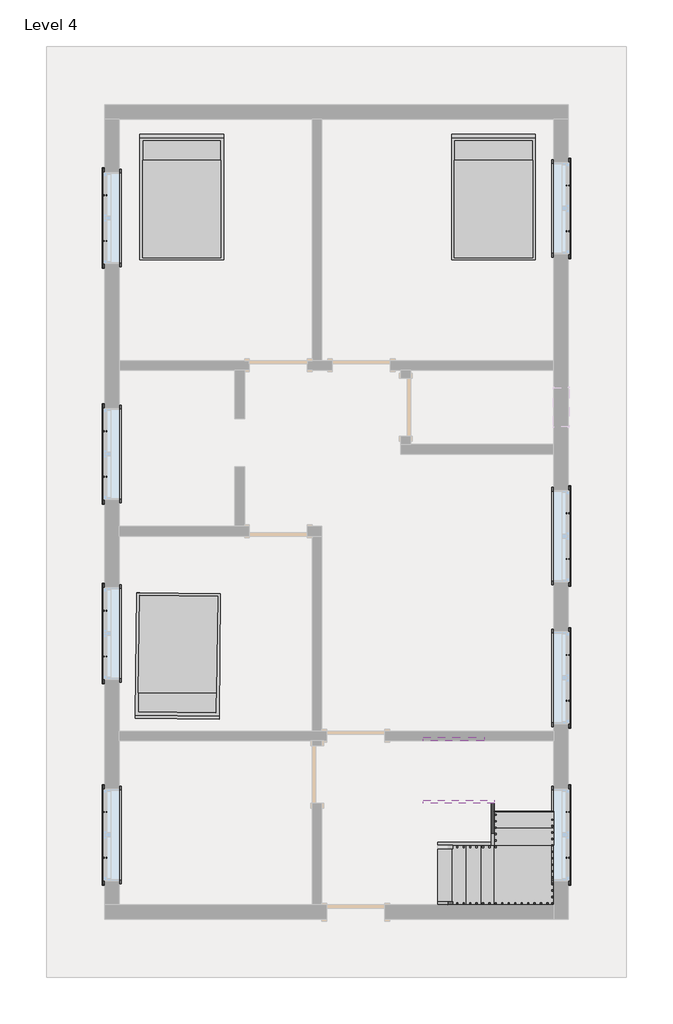
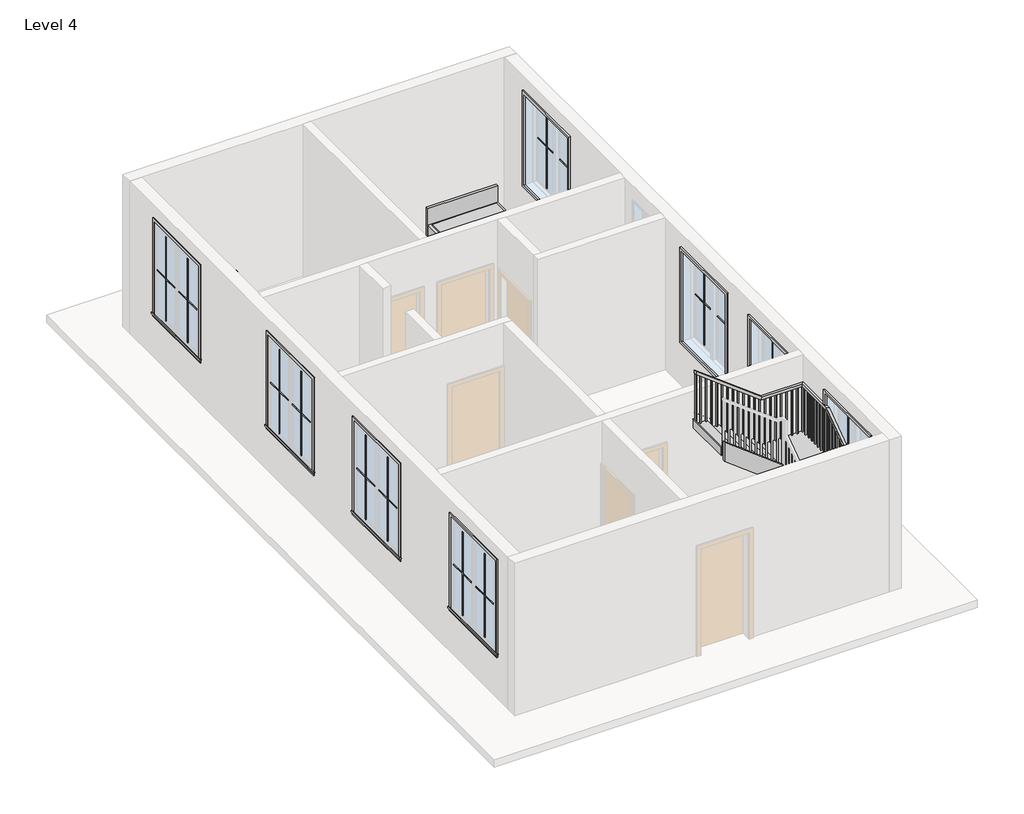
# One storey, part 2 of 2: 32 proxies, 5 members, 3 furniture elements, 1 railing, 1 stair flight.
"""IFC4 building model written with IfcOpenShell, lengths in millimetres."""

from ifc_helpers import new_model, si_unit, frame, origin, place, context, project, spatial, polyline, outline, extrude, faceted_brep, transform, mapped, element, save
from components import muntin_pattern_2x2_muntin_pattern_2x2_bff912c5, muntin_pattern_2x2_muntin_pattern_2x2_c2194282, trim_window_exterior_flat_with_sill_e04b3088, trim_window_interior_flat_picture_frame_2a7685fe, bed_17739_bed_17739_15c61121, stair_flight_c7955c98

model = new_model("IFC4")

# Units and contexts
model_context = context("Model", 3, world=origin())
ifc_project = project(units=[si_unit("LENGTHUNIT", "METRE", prefix="MILLI")], contexts=[model_context])

# Site, building, storey
site = spatial("IfcSite", under=ifc_project)
building = spatial("IfcBuilding", under=site)
storey = spatial("IfcBuildingStorey", under=building, Name="Level 4", Elevation=6400.8)

# Proxies
placement = place(None, origin())
muntin_pattern_2x2_muntin_pattern_2x2_shape = muntin_pattern_2x2_muntin_pattern_2x2_bff912c5(model_context)
element("IfcBuildingElementProxy", 1, Name="Muntin Pattern_2x2 : Muntin Pattern_2x2", ObjectType="Muntin Pattern_2x2 : Muntin Pattern_2x2", at=placement, inside=storey, context=model_context, shape_type="MappedRepresentation", body=[
    mapped(muntin_pattern_2x2_muntin_pattern_2x2_shape, transform((-4903.510885, -5396.5975571, 7385.05), x_axis=(0.0, 1.0, 0.0), y_axis=(-1.0, 0.0, 0.0), z_axis=(0.0, 0.0, 1.0))),
])
element("IfcBuildingElementProxy", 2, Name="Muntin Pattern_2x2 : Muntin Pattern_2x2", ObjectType="Muntin Pattern_2x2 : Muntin Pattern_2x2", at=placement, inside=storey, context=model_context, shape_type="MappedRepresentation", body=[
    mapped(muntin_pattern_2x2_muntin_pattern_2x2_shape, transform((2392.639115, -4675.8725571, 7385.05), x_axis=(0.0, -1.0, 0.0), y_axis=(1.0, 0.0, 0.0), z_axis=(0.0, 0.0, 1.0))),
])
element("IfcBuildingElementProxy", 3, Name="Muntin Pattern_2x2 : Muntin Pattern_2x2", ObjectType="Muntin Pattern_2x2 : Muntin Pattern_2x2", at=placement, inside=storey, context=model_context, shape_type="MappedRepresentation", body=[
    mapped(muntin_pattern_2x2_muntin_pattern_2x2_shape, transform((2392.639115, -2199.3725571, 7385.05), x_axis=(0.0, -1.0, 0.0), y_axis=(1.0, 0.0, 0.0), z_axis=(0.0, 0.0, 1.0))),
])
element("IfcBuildingElementProxy", 4, Name="Muntin Pattern_2x2 : Muntin Pattern_2x2", ObjectType="Muntin Pattern_2x2 : Muntin Pattern_2x2", at=placement, inside=storey, context=model_context, shape_type="MappedRepresentation", body=[
    mapped(muntin_pattern_2x2_muntin_pattern_2x2_shape, transform((2392.639115, 35.8274429, 7385.05), x_axis=(0.0, -1.0, 0.0), y_axis=(1.0, 0.0, 0.0), z_axis=(0.0, 0.0, 1.0))),
])
element("IfcBuildingElementProxy", 5, Name="Muntin Pattern_2x2 : Muntin Pattern_2x2", ObjectType="Muntin Pattern_2x2 : Muntin Pattern_2x2", at=placement, inside=storey, context=model_context, shape_type="MappedRepresentation", body=[
    mapped(muntin_pattern_2x2_muntin_pattern_2x2_shape, transform((-4903.510885, -2221.5975571, 7385.05), x_axis=(0.0, 1.0, 0.0), y_axis=(-1.0, 0.0, 0.0), z_axis=(0.0, 0.0, 1.0))),
])
element("IfcBuildingElementProxy", 6, Name="Muntin Pattern_2x2 : Muntin Pattern_2x2", ObjectType="Muntin Pattern_2x2 : Muntin Pattern_2x2", at=placement, inside=storey, context=model_context, shape_type="MappedRepresentation", body=[
    mapped(muntin_pattern_2x2_muntin_pattern_2x2_shape, transform((-4903.510885, 610.5024429, 7385.05), x_axis=(0.0, 1.0, 0.0), y_axis=(-1.0, 0.0, 0.0), z_axis=(0.0, 0.0, 1.0))),
])
element("IfcBuildingElementProxy", 7, Name="Muntin Pattern_2x2 : Muntin Pattern_2x2", ObjectType="Muntin Pattern_2x2 : Muntin Pattern_2x2", at=placement, inside=storey, context=model_context, shape_type="MappedRepresentation", body=[
    mapped(muntin_pattern_2x2_muntin_pattern_2x2_shape, transform((-4903.510885, 4331.6024429, 7385.05), x_axis=(0.0, 1.0, 0.0), y_axis=(-1.0, 0.0, 0.0), z_axis=(0.0, 0.0, 1.0))),
])
element("IfcBuildingElementProxy", 8, Name="Muntin Pattern_2x2 : Muntin Pattern_2x2", ObjectType="Muntin Pattern_2x2 : Muntin Pattern_2x2", at=placement, inside=storey, context=model_context, shape_type="MappedRepresentation", body=[
    mapped(muntin_pattern_2x2_muntin_pattern_2x2_shape, transform((2392.639115, 5204.7274429, 7385.05), x_axis=(0.0, -1.0, 0.0), y_axis=(1.0, 0.0, 0.0), z_axis=(0.0, 0.0, 1.0))),
])
muntin_pattern_2x2_muntin_pattern_2x2_2_shape = muntin_pattern_2x2_muntin_pattern_2x2_c2194282(model_context)
element("IfcBuildingElementProxy", 9, Name="Muntin Pattern_2x2 : Muntin Pattern_2x2", ObjectType="Muntin Pattern_2x2 : Muntin Pattern_2x2", at=placement, inside=storey, context=model_context, shape_type="MappedRepresentation", body=[
    mapped(muntin_pattern_2x2_muntin_pattern_2x2_2_shape, transform((-4903.510885, -4675.8725571, 7385.05), x_axis=(0.0, -1.0, 0.0), y_axis=(1.0, 0.0, 0.0), z_axis=(0.0, 0.0, 1.0))),
])
element("IfcBuildingElementProxy", 10, Name="Muntin Pattern_2x2 : Muntin Pattern_2x2", ObjectType="Muntin Pattern_2x2 : Muntin Pattern_2x2", at=placement, inside=storey, context=model_context, shape_type="MappedRepresentation", body=[
    mapped(muntin_pattern_2x2_muntin_pattern_2x2_2_shape, transform((2392.639115, -5396.5975571, 7385.05), x_axis=(0.0, 1.0, 0.0), y_axis=(-1.0, 0.0, 0.0), z_axis=(0.0, 0.0, 1.0))),
])
element("IfcBuildingElementProxy", 11, Name="Muntin Pattern_2x2 : Muntin Pattern_2x2", ObjectType="Muntin Pattern_2x2 : Muntin Pattern_2x2", at=placement, inside=storey, context=model_context, shape_type="MappedRepresentation", body=[
    mapped(muntin_pattern_2x2_muntin_pattern_2x2_2_shape, transform((2392.639115, -2920.0975571, 7385.05), x_axis=(0.0, 1.0, 0.0), y_axis=(-1.0, 0.0, 0.0), z_axis=(0.0, 0.0, 1.0))),
])
element("IfcBuildingElementProxy", 12, Name="Muntin Pattern_2x2 : Muntin Pattern_2x2", ObjectType="Muntin Pattern_2x2 : Muntin Pattern_2x2", at=placement, inside=storey, context=model_context, shape_type="MappedRepresentation", body=[
    mapped(muntin_pattern_2x2_muntin_pattern_2x2_2_shape, transform((2392.639115, -684.8975571, 7385.05), x_axis=(0.0, 1.0, 0.0), y_axis=(-1.0, 0.0, 0.0), z_axis=(0.0, 0.0, 1.0))),
])
element("IfcBuildingElementProxy", 13, Name="Muntin Pattern_2x2 : Muntin Pattern_2x2", ObjectType="Muntin Pattern_2x2 : Muntin Pattern_2x2", at=placement, inside=storey, context=model_context, shape_type="MappedRepresentation", body=[
    mapped(muntin_pattern_2x2_muntin_pattern_2x2_2_shape, transform((-4903.510885, -1500.8725571, 7385.05), x_axis=(0.0, -1.0, 0.0), y_axis=(1.0, 0.0, 0.0), z_axis=(0.0, 0.0, 1.0))),
])
element("IfcBuildingElementProxy", 14, Name="Muntin Pattern_2x2 : Muntin Pattern_2x2", ObjectType="Muntin Pattern_2x2 : Muntin Pattern_2x2", at=placement, inside=storey, context=model_context, shape_type="MappedRepresentation", body=[
    mapped(muntin_pattern_2x2_muntin_pattern_2x2_2_shape, transform((-4903.510885, 1331.2274429, 7385.05), x_axis=(0.0, -1.0, 0.0), y_axis=(1.0, 0.0, 0.0), z_axis=(0.0, 0.0, 1.0))),
])
element("IfcBuildingElementProxy", 15, Name="Muntin Pattern_2x2 : Muntin Pattern_2x2", ObjectType="Muntin Pattern_2x2 : Muntin Pattern_2x2", at=placement, inside=storey, context=model_context, shape_type="MappedRepresentation", body=[
    mapped(muntin_pattern_2x2_muntin_pattern_2x2_2_shape, transform((-4903.510885, 5052.3274429, 7385.05), x_axis=(0.0, -1.0, 0.0), y_axis=(1.0, 0.0, 0.0), z_axis=(0.0, 0.0, 1.0))),
])
element("IfcBuildingElementProxy", 16, Name="Muntin Pattern_2x2 : Muntin Pattern_2x2", ObjectType="Muntin Pattern_2x2 : Muntin Pattern_2x2", at=placement, inside=storey, context=model_context, shape_type="MappedRepresentation", body=[
    mapped(muntin_pattern_2x2_muntin_pattern_2x2_2_shape, transform((2392.639115, 4484.0024429, 7385.05), x_axis=(0.0, 1.0, 0.0), y_axis=(-1.0, 0.0, 0.0), z_axis=(0.0, 0.0, 1.0))),
])
trim_window_exterior_flat_with_sill_shape = trim_window_exterior_flat_with_sill_e04b3088(model_context)
element("IfcBuildingElementProxy", 17, Name="Trim-Window-Exterior-Flat : with Sill", ObjectType="Trim-Window-Exterior-Flat : with Sill", at=placement, inside=storey, context=model_context, shape_type="MappedRepresentation", body=[
    mapped(trim_window_exterior_flat_with_sill_shape, transform((-4913.035885, -5036.2350571, 9144.0), x_axis=(0.0, -1.0, 0.0), y_axis=(0.0, 0.0, 1.0), z_axis=(-1.0, 0.0, 0.0))),
])
element("IfcBuildingElementProxy", 18, Name="Trim-Window-Exterior-Flat : with Sill", ObjectType="Trim-Window-Exterior-Flat : with Sill", at=placement, inside=storey, context=model_context, shape_type="MappedRepresentation", body=[
    mapped(trim_window_exterior_flat_with_sill_shape, transform((2402.164115, -5036.2350571, 9144.0), x_axis=(0.0, 1.0, 0.0), y_axis=(0.0, 0.0, 1.0), z_axis=(1.0, 0.0, 0.0))),
])
element("IfcBuildingElementProxy", 19, Name="Trim-Window-Exterior-Flat : with Sill", ObjectType="Trim-Window-Exterior-Flat : with Sill", at=placement, inside=storey, context=model_context, shape_type="MappedRepresentation", body=[
    mapped(trim_window_exterior_flat_with_sill_shape, transform((2402.164115, -2559.7350571, 9144.0), x_axis=(0.0, 1.0, 0.0), y_axis=(0.0, 0.0, 1.0), z_axis=(1.0, 0.0, 0.0))),
])
element("IfcBuildingElementProxy", 20, Name="Trim-Window-Exterior-Flat : with Sill", ObjectType="Trim-Window-Exterior-Flat : with Sill", at=placement, inside=storey, context=model_context, shape_type="MappedRepresentation", body=[
    mapped(trim_window_exterior_flat_with_sill_shape, transform((2402.164115, -324.5350571, 9144.0), x_axis=(0.0, 1.0, 0.0), y_axis=(0.0, 0.0, 1.0), z_axis=(1.0, 0.0, 0.0))),
])
element("IfcBuildingElementProxy", 21, Name="Trim-Window-Exterior-Flat : with Sill", ObjectType="Trim-Window-Exterior-Flat : with Sill", at=placement, inside=storey, context=model_context, shape_type="MappedRepresentation", body=[
    mapped(trim_window_exterior_flat_with_sill_shape, transform((-4913.035885, -1861.2350571, 9144.0), x_axis=(0.0, -1.0, 0.0), y_axis=(0.0, 0.0, 1.0), z_axis=(-1.0, 0.0, 0.0))),
])
element("IfcBuildingElementProxy", 22, Name="Trim-Window-Exterior-Flat : with Sill", ObjectType="Trim-Window-Exterior-Flat : with Sill", at=placement, inside=storey, context=model_context, shape_type="MappedRepresentation", body=[
    mapped(trim_window_exterior_flat_with_sill_shape, transform((-4913.035885, 970.8649429, 9144.0), x_axis=(0.0, -1.0, 0.0), y_axis=(0.0, 0.0, 1.0), z_axis=(-1.0, 0.0, 0.0))),
])
element("IfcBuildingElementProxy", 23, Name="Trim-Window-Exterior-Flat : with Sill", ObjectType="Trim-Window-Exterior-Flat : with Sill", at=placement, inside=storey, context=model_context, shape_type="MappedRepresentation", body=[
    mapped(trim_window_exterior_flat_with_sill_shape, transform((-4913.035885, 4691.9649429, 9144.0), x_axis=(0.0, -1.0, 0.0), y_axis=(0.0, 0.0, 1.0), z_axis=(-1.0, 0.0, 0.0))),
])
element("IfcBuildingElementProxy", 24, Name="Trim-Window-Exterior-Flat : with Sill", ObjectType="Trim-Window-Exterior-Flat : with Sill", at=placement, inside=storey, context=model_context, shape_type="MappedRepresentation", body=[
    mapped(trim_window_exterior_flat_with_sill_shape, transform((2402.164115, 4844.3649429, 9144.0), x_axis=(0.0, 1.0, 0.0), y_axis=(0.0, 0.0, 1.0), z_axis=(1.0, 0.0, 0.0))),
])
trim_window_interior_flat_picture_frame_shape = trim_window_interior_flat_picture_frame_2a7685fe(model_context)
element("IfcBuildingElementProxy", 25, Name="Trim-Window-Interior-Flat : Picture Frame", ObjectType="Trim-Window-Interior-Flat : Picture Frame", at=placement, inside=storey, context=model_context, shape_type="MappedRepresentation", body=[
    mapped(trim_window_interior_flat_picture_frame_shape, transform((-4684.435885, -5036.2350571, 9144.0), x_axis=(0.0, 1.0, 0.0), y_axis=(0.0, 0.0, 1.0), z_axis=(1.0, 0.0, 0.0))),
])
element("IfcBuildingElementProxy", 26, Name="Trim-Window-Interior-Flat : Picture Frame", ObjectType="Trim-Window-Interior-Flat : Picture Frame", at=placement, inside=storey, context=model_context, shape_type="MappedRepresentation", body=[
    mapped(trim_window_interior_flat_picture_frame_shape, transform((2173.564115, -5036.2350571, 9144.0), x_axis=(0.0, -1.0, 0.0), y_axis=(0.0, 0.0, 1.0), z_axis=(-1.0, 0.0, 0.0))),
])
element("IfcBuildingElementProxy", 27, Name="Trim-Window-Interior-Flat : Picture Frame", ObjectType="Trim-Window-Interior-Flat : Picture Frame", at=placement, inside=storey, context=model_context, shape_type="MappedRepresentation", body=[
    mapped(trim_window_interior_flat_picture_frame_shape, transform((2173.564115, -2559.7350571, 9144.0), x_axis=(0.0, -1.0, 0.0), y_axis=(0.0, 0.0, 1.0), z_axis=(-1.0, 0.0, 0.0))),
])
element("IfcBuildingElementProxy", 28, Name="Trim-Window-Interior-Flat : Picture Frame", ObjectType="Trim-Window-Interior-Flat : Picture Frame", at=placement, inside=storey, context=model_context, shape_type="MappedRepresentation", body=[
    mapped(trim_window_interior_flat_picture_frame_shape, transform((2173.564115, -324.5350571, 9144.0), x_axis=(0.0, -1.0, 0.0), y_axis=(0.0, 0.0, 1.0), z_axis=(-1.0, 0.0, 0.0))),
])
element("IfcBuildingElementProxy", 29, Name="Trim-Window-Interior-Flat : Picture Frame", ObjectType="Trim-Window-Interior-Flat : Picture Frame", at=placement, inside=storey, context=model_context, shape_type="MappedRepresentation", body=[
    mapped(trim_window_interior_flat_picture_frame_shape, transform((-4684.435885, -1861.2350571, 9144.0), x_axis=(0.0, 1.0, 0.0), y_axis=(0.0, 0.0, 1.0), z_axis=(1.0, 0.0, 0.0))),
])
element("IfcBuildingElementProxy", 30, Name="Trim-Window-Interior-Flat : Picture Frame", ObjectType="Trim-Window-Interior-Flat : Picture Frame", at=placement, inside=storey, context=model_context, shape_type="MappedRepresentation", body=[
    mapped(trim_window_interior_flat_picture_frame_shape, transform((-4684.435885, 970.8649429, 9144.0), x_axis=(0.0, 1.0, 0.0), y_axis=(0.0, 0.0, 1.0), z_axis=(1.0, 0.0, 0.0))),
])
element("IfcBuildingElementProxy", 31, Name="Trim-Window-Interior-Flat : Picture Frame", ObjectType="Trim-Window-Interior-Flat : Picture Frame", at=placement, inside=storey, context=model_context, shape_type="MappedRepresentation", body=[
    mapped(trim_window_interior_flat_picture_frame_shape, transform((-4684.435885, 4691.9649429, 9144.0), x_axis=(0.0, 1.0, 0.0), y_axis=(0.0, 0.0, 1.0), z_axis=(1.0, 0.0, 0.0))),
])
element("IfcBuildingElementProxy", 32, Name="Trim-Window-Interior-Flat : Picture Frame", ObjectType="Trim-Window-Interior-Flat : Picture Frame", at=placement, inside=storey, context=model_context, shape_type="MappedRepresentation", body=[
    mapped(trim_window_interior_flat_picture_frame_shape, transform((2173.564115, 4844.3649429, 9144.0), x_axis=(0.0, -1.0, 0.0), y_axis=(0.0, 0.0, 1.0), z_axis=(-1.0, 0.0, 0.0))),
])

# Furniture
bed_17739_bed_17739_shape = bed_17739_bed_17739_15c61121(model_context)
element("IfcFurniture", 33, ObjectType="Bed_17739 : Bed_17739", at=placement, inside=storey, context=model_context, shape_type="MappedRepresentation", body=[
    mapped(bed_17739_bed_17739_shape, transform((-3693.835885, 4996.7649429, 6400.8), x_axis=(1.0, 0.0, 0.0), y_axis=(0.0, 1.0, 0.0), z_axis=(0.0, 0.0, 1.0))),
])
element("IfcFurniture", 34, ObjectType="Bed_17739 : Bed_17739", at=placement, inside=storey, context=model_context, shape_type="MappedRepresentation", body=[
    mapped(bed_17739_bed_17739_shape, transform((1221.064115, 4996.7649429, 6400.8), x_axis=(1.0, 0.0, 0.0), y_axis=(0.0, 1.0, 0.0), z_axis=(0.0, 0.0, 1.0))),
])
element("IfcFurniture", 35, ObjectType="Bed_17739 : Bed_17739", at=placement, inside=storey, context=model_context, shape_type="MappedRepresentation", body=[
    mapped(bed_17739_bed_17739_shape, transform((-3756.0321663, -2189.364606, 6400.8), x_axis=(-0.9999334593473937, 0.011535895177843815, 0.0), y_axis=(-0.011535895177843815, -0.9999334593473937, 0.0), z_axis=(0.0, 0.0, 1.0))),
])

# Members
element("IfcMember", 36, ObjectType="Stringer - 2\" Width", at=placement, inside=storey, context=model_context, shape_type="SweptSolid", body=[
    extrude(outline(polyline([(6623.4959685, 344.764115), (6400.8, 344.764115), (6400.8, 555.1685253), (6883.7196844, 1182.964115), (7268.2651993, 1182.964115), (6623.4959685, 344.764115)])), frame((0.0, -5201.3350571, 0.0), z_axis=(0.0, 1.0, 0.0), x_axis=(0.0, 0.0, 1.0)), (0.0, 0.0, 1.0), 50.8),
])
element("IfcMember", 37, ObjectType="Stringer - 2\" Width", at=placement, inside=storey, context=model_context, shape_type="SweptSolid", body=[
    extrude(outline(polyline([(-5201.3350571, 7095.952716), (-5201.3350571, 7470.5225362), (-4540.9350571, 7942.2368219), (-4540.9350571, 7567.6670017), (-5201.3350571, 7095.952716)])), frame((1182.964115, 0.0, 0.0), z_axis=(1.0, 0.0, 0.0), x_axis=(0.0, 1.0, 0.0)), (0.0, 0.0, 1.0), 50.8),
])
element("IfcMember", 38, ObjectType="Stringer - 2\" Width", at=placement, inside=storey, context=model_context, shape_type="SweptSolid", body=[
    extrude(outline(polyline([(7769.9786616, 1233.764115), (8153.1668, 1233.764115), (9004.6715619, 116.164115), (8621.4834236, 116.164115), (7769.9786616, 1233.764115)])), frame((0.0, -4540.9350571, 0.0), z_axis=(0.0, 1.0, 0.0), x_axis=(0.0, 0.0, 1.0)), (0.0, 0.0, 1.0), 50.8),
])
element("IfcMember", 39, ObjectType="Stringer - 2\" Width", at=placement, inside=storey, context=model_context, shape_type="SweptSolid", body=[
    extrude(outline(polyline([(6623.4959685, 344.764115), (6400.8, 344.764115), (6400.8, 555.1685253), (6799.2368219, 1073.1363938), (6799.2368219, 573.2272245), (6623.4959685, 344.764115)])), frame((0.0, -6191.9350571, 0.0), z_axis=(0.0, 1.0, 0.0), x_axis=(0.0, 0.0, 1.0)), (0.0, 0.0, 1.0), 50.8),
])
element("IfcMember", 40, ObjectType="Stringer - 2\" Width", at=placement, inside=storey, context=model_context, shape_type="SweptSolid", body=[
    extrude(outline(polyline([(8275.2384303, 1073.5451003), (9004.6715619, 116.164115), (8621.4834236, 116.164115), (8275.2384303, 570.6106687), (8275.2384303, 1073.5451003)])), frame((0.0, -3550.3350571, 0.0), z_axis=(0.0, 1.0, 0.0), x_axis=(0.0, 0.0, 1.0)), (0.0, 0.0, 1.0), 50.8),
])

# Railing
element("IfcRailing", 41, ObjectType="Handrail - Rectangular", at=placement, inside=storey, context=model_context, shape_type="SolidModel", body=[
    faceted_brep([(344.764115, -6090.3350571, 7484.5333333), (344.764115, -6090.3350571, 7420.6686436), (344.764115, -6141.1350571, 7420.6686436), (344.764115, -6141.1350571, 7484.5333333), (1373.464115, -6090.3350571, 8268.3047619), (1390.6115203, -6090.3350571, 8217.5047619), (1390.6115203, -6141.1350571, 8217.5047619), (1373.464115, -6141.1350571, 8268.3047619), (2122.764115, -6090.3350571, 8268.3047619), (2122.764115, -6090.3350571, 8217.5047619), (2173.564115, -6141.1350571, 8217.5047619), (2173.564115, -6141.1350571, 8268.3047619), (2122.764115, -5289.3883904, 8268.3047619), (2122.764115, -5273.1087657, 8217.5047619), (2173.564115, -5273.1087657, 8217.5047619), (2173.564115, -5289.3883904, 8268.3047619), (2122.764115, -4399.3108146, 8904.0744589), (2122.764115, -4383.0311899, 8853.2744589), (2173.564115, -4383.0311899, 8853.2744589), (2173.564115, -4399.3108146, 8904.0744589), (2122.764115, -3601.1350571, 8904.0744589), (2122.764115, -3601.1350571, 8853.2744589), (2173.564115, -3550.3350571, 8853.2744589), (2173.564115, -3550.3350571, 8904.0744589), (1371.6498293, -3601.1350571, 8904.0744589), (1354.5800477, -3601.1350571, 8853.2744589), (1354.5800477, -3550.3350571, 8853.2744589), (1371.6498293, -3550.3350571, 8904.0744589), (116.164115, -3601.1350571, 9855.2), (116.164115, -3550.3350571, 9855.2), (116.164115, -3550.3350571, 9791.4683472), (116.164115, -3601.1350571, 9791.4683472)], [[[0, 1, 2, 3]], [[1, 0, 4, 5]], [[2, 1, 5, 6]], [[3, 2, 6, 7]], [[0, 3, 7, 4]], [[5, 4, 8, 9]], [[6, 5, 9, 10]], [[7, 6, 10, 11]], [[4, 7, 11, 8]], [[9, 8, 12, 13]], [[10, 9, 13, 14]], [[11, 10, 14, 15]], [[8, 11, 15, 12]], [[13, 12, 16, 17]], [[14, 13, 17, 18]], [[15, 14, 18, 19]], [[12, 15, 19, 16]], [[17, 16, 20, 21]], [[18, 17, 21, 22]], [[19, 18, 22, 23]], [[16, 19, 23, 20]], [[21, 20, 24, 25]], [[22, 21, 25, 26]], [[23, 22, 26, 27]], [[20, 23, 27, 24]], [[28, 29, 30, 31]], [[25, 24, 28, 31]], [[26, 25, 31, 30]], [[27, 26, 30, 29]], [[24, 27, 29, 28]]]),
    extrude(outline(polyline([(9707.2827412, 227.289115), (9721.7145594, 208.239115), (8771.4666667, 208.239115), (8771.4666667, 227.289115), (9707.2827412, 227.289115)])), frame((0.0, -3585.2600571, 0.0), z_axis=(0.0, 1.0, 0.0), x_axis=(0.0, 0.0, 1.0)), (0.0, 0.0, 1.0), 19.05),
    extrude(outline(polyline([(9630.3130442, 328.889115), (9644.7448624, 309.839115), (8771.4666667, 309.839115), (8771.4666667, 328.889115), (9630.3130442, 328.889115)])), frame((0.0, -3585.2600571, 0.0), z_axis=(0.0, 1.0, 0.0), x_axis=(0.0, 0.0, 1.0)), (0.0, 0.0, 1.0), 19.05),
    extrude(outline(polyline([(9553.3433472, 430.489115), (9567.7751654, 411.439115), (8602.1333333, 411.439115), (8602.1333333, 430.489115), (9553.3433472, 430.489115)])), frame((0.0, -3585.2600571, 0.0), z_axis=(0.0, 1.0, 0.0), x_axis=(0.0, 0.0, 1.0)), (0.0, 0.0, 1.0), 19.05),
    extrude(outline(polyline([(9476.3736503, 532.089115), (9490.8054685, 513.039115), (8602.1333333, 513.039115), (8602.1333333, 532.089115), (9476.3736503, 532.089115)])), frame((0.0, -3585.2600571, 0.0), z_axis=(0.0, 1.0, 0.0), x_axis=(0.0, 0.0, 1.0)), (0.0, 0.0, 1.0), 19.05),
    extrude(outline(polyline([(9399.4039533, 633.689115), (9413.8357715, 614.639115), (8432.8, 614.639115), (8432.8, 633.689115), (9399.4039533, 633.689115)])), frame((0.0, -3585.2600571, 0.0), z_axis=(0.0, 1.0, 0.0), x_axis=(0.0, 0.0, 1.0)), (0.0, 0.0, 1.0), 19.05),
    extrude(outline(polyline([(9322.4342563, 735.289115), (9336.8660745, 716.239115), (8432.8, 716.239115), (8432.8, 735.289115), (9322.4342563, 735.289115)])), frame((0.0, -3585.2600571, 0.0), z_axis=(0.0, 1.0, 0.0), x_axis=(0.0, 0.0, 1.0)), (0.0, 0.0, 1.0), 19.05),
    extrude(outline(polyline([(9245.4645594, 836.889115), (9259.8963775, 817.839115), (8263.4666667, 817.839115), (8263.4666667, 836.889115), (9245.4645594, 836.889115)])), frame((0.0, -3585.2600571, 0.0), z_axis=(0.0, 1.0, 0.0), x_axis=(0.0, 0.0, 1.0)), (0.0, 0.0, 1.0), 19.05),
    extrude(outline(polyline([(9168.4948624, 938.489115), (9182.9266806, 919.439115), (8263.4666667, 919.439115), (8263.4666667, 938.489115), (9168.4948624, 938.489115)])), frame((0.0, -3585.2600571, 0.0), z_axis=(0.0, 1.0, 0.0), x_axis=(0.0, 0.0, 1.0)), (0.0, 0.0, 1.0), 19.05),
    extrude(outline(polyline([(9091.5251654, 1040.089115), (9105.9569836, 1021.039115), (8263.4666667, 1021.039115), (8263.4666667, 1040.089115), (9091.5251654, 1040.089115)])), frame((0.0, -3585.2600571, 0.0), z_axis=(0.0, 1.0, 0.0), x_axis=(0.0, 0.0, 1.0)), (0.0, 0.0, 1.0), 19.05),
    extrude(outline(polyline([(9014.5554685, 1141.689115), (9028.9872866, 1122.639115), (8094.1333333, 1122.639115), (8094.1333333, 1141.689115), (9014.5554685, 1141.689115)])), frame((0.0, -3585.2600571, 0.0), z_axis=(0.0, 1.0, 0.0), x_axis=(0.0, 0.0, 1.0)), (0.0, 0.0, 1.0), 19.05),
    extrude(outline(polyline([(8937.5857715, 1243.289115), (8952.0175897, 1224.239115), (8094.1333333, 1224.239115), (8094.1333333, 1243.289115), (8937.5857715, 1243.289115)])), frame((0.0, -3585.2600571, 0.0), z_axis=(0.0, 1.0, 0.0), x_axis=(0.0, 0.0, 1.0)), (0.0, 0.0, 1.0), 19.05),
    extrude(outline(polyline([(8860.6160745, 1344.889115), (8875.0478927, 1325.839115), (7924.8, 1325.839115), (7924.8, 1344.889115), (8860.6160745, 1344.889115)])), frame((0.0, -3585.2600571, 0.0), z_axis=(0.0, 1.0, 0.0), x_axis=(0.0, 0.0, 1.0)), (0.0, 0.0, 1.0), 19.05),
    extrude(outline(polyline([(1446.489115, -3566.2100571), (1446.489115, -3585.2600571), (1427.439115, -3585.2600571), (1427.439115, -3566.2100571), (1446.489115, -3566.2100571)])), frame((0.0, 0.0, 7924.8), z_axis=(0.0, 0.0, 1.0), x_axis=(1.0, 0.0, 0.0)), (0.0, 0.0, 1.0), 928.4744589),
    extrude(outline(polyline([(1548.089115, -3566.2100571), (1548.089115, -3585.2600571), (1529.039115, -3585.2600571), (1529.039115, -3566.2100571), (1548.089115, -3566.2100571)])), frame((0.0, 0.0, 7924.8), z_axis=(0.0, 0.0, 1.0), x_axis=(1.0, 0.0, 0.0)), (0.0, 0.0, 1.0), 928.4744589),
    extrude(outline(polyline([(1649.689115, -3566.2100571), (1649.689115, -3585.2600571), (1630.639115, -3585.2600571), (1630.639115, -3566.2100571), (1649.689115, -3566.2100571)])), frame((0.0, 0.0, 7924.8), z_axis=(0.0, 0.0, 1.0), x_axis=(1.0, 0.0, 0.0)), (0.0, 0.0, 1.0), 928.4744589),
    extrude(outline(polyline([(1751.289115, -3566.2100571), (1751.289115, -3585.2600571), (1732.239115, -3585.2600571), (1732.239115, -3566.2100571), (1751.289115, -3566.2100571)])), frame((0.0, 0.0, 7924.8), z_axis=(0.0, 0.0, 1.0), x_axis=(1.0, 0.0, 0.0)), (0.0, 0.0, 1.0), 928.4744589),
    extrude(outline(polyline([(1852.889115, -3566.2100571), (1852.889115, -3585.2600571), (1833.839115, -3585.2600571), (1833.839115, -3566.2100571), (1852.889115, -3566.2100571)])), frame((0.0, 0.0, 7924.8), z_axis=(0.0, 0.0, 1.0), x_axis=(1.0, 0.0, 0.0)), (0.0, 0.0, 1.0), 928.4744589),
    extrude(outline(polyline([(1954.489115, -3566.2100571), (1954.489115, -3585.2600571), (1935.439115, -3585.2600571), (1935.439115, -3566.2100571), (1954.489115, -3566.2100571)])), frame((0.0, 0.0, 7924.8), z_axis=(0.0, 0.0, 1.0), x_axis=(1.0, 0.0, 0.0)), (0.0, 0.0, 1.0), 928.4744589),
    extrude(outline(polyline([(2056.089115, -3566.2100571), (2056.089115, -3585.2600571), (2037.039115, -3585.2600571), (2037.039115, -3566.2100571), (2056.089115, -3566.2100571)])), frame((0.0, 0.0, 7924.8), z_axis=(0.0, 0.0, 1.0), x_axis=(1.0, 0.0, 0.0)), (0.0, 0.0, 1.0), 928.4744589),
    extrude(outline(polyline([(2157.689115, -3686.8600571), (2138.639115, -3686.8600571), (2138.639115, -3667.8100571), (2157.689115, -3667.8100571), (2157.689115, -3686.8600571)])), frame((0.0, 0.0, 7924.8), z_axis=(0.0, 0.0, 1.0), x_axis=(1.0, 0.0, 0.0)), (0.0, 0.0, 1.0), 928.4744589),
    extrude(outline(polyline([(2157.689115, -3788.4600571), (2138.639115, -3788.4600571), (2138.639115, -3769.4100571), (2157.689115, -3769.4100571), (2157.689115, -3788.4600571)])), frame((0.0, 0.0, 7924.8), z_axis=(0.0, 0.0, 1.0), x_axis=(1.0, 0.0, 0.0)), (0.0, 0.0, 1.0), 928.4744589),
    extrude(outline(polyline([(2157.689115, -3890.0600571), (2138.639115, -3890.0600571), (2138.639115, -3871.0100571), (2157.689115, -3871.0100571), (2157.689115, -3890.0600571)])), frame((0.0, 0.0, 7924.8), z_axis=(0.0, 0.0, 1.0), x_axis=(1.0, 0.0, 0.0)), (0.0, 0.0, 1.0), 928.4744589),
    extrude(outline(polyline([(2157.689115, -3991.6600571), (2138.639115, -3991.6600571), (2138.639115, -3972.6100571), (2157.689115, -3972.6100571), (2157.689115, -3991.6600571)])), frame((0.0, 0.0, 7924.8), z_axis=(0.0, 0.0, 1.0), x_axis=(1.0, 0.0, 0.0)), (0.0, 0.0, 1.0), 928.4744589),
    extrude(outline(polyline([(2157.689115, -4093.2600571), (2138.639115, -4093.2600571), (2138.639115, -4074.2100571), (2157.689115, -4074.2100571), (2157.689115, -4093.2600571)])), frame((0.0, 0.0, 7924.8), z_axis=(0.0, 0.0, 1.0), x_axis=(1.0, 0.0, 0.0)), (0.0, 0.0, 1.0), 928.4744589),
    extrude(outline(polyline([(2157.689115, -4194.8600571), (2138.639115, -4194.8600571), (2138.639115, -4175.8100571), (2157.689115, -4175.8100571), (2157.689115, -4194.8600571)])), frame((0.0, 0.0, 7924.8), z_axis=(0.0, 0.0, 1.0), x_axis=(1.0, 0.0, 0.0)), (0.0, 0.0, 1.0), 928.4744589),
    extrude(outline(polyline([(2157.689115, -4296.4600571), (2138.639115, -4296.4600571), (2138.639115, -4277.4100571), (2157.689115, -4277.4100571), (2157.689115, -4296.4600571)])), frame((0.0, 0.0, 7924.8), z_axis=(0.0, 0.0, 1.0), x_axis=(1.0, 0.0, 0.0)), (0.0, 0.0, 1.0), 928.4744589),
    extrude(outline(polyline([(2157.689115, -4398.0600571), (2138.639115, -4398.0600571), (2138.639115, -4379.0100571), (2157.689115, -4379.0100571), (2157.689115, -4398.0600571)])), frame((0.0, 0.0, 7924.8), z_axis=(0.0, 0.0, 1.0), x_axis=(1.0, 0.0, 0.0)), (0.0, 0.0, 1.0), 928.4744589),
    extrude(outline(polyline([(-4499.6600571, 8769.9681252), (-4480.6100571, 8783.5752681), (-4480.6100571, 7924.8), (-4499.6600571, 7924.8), (-4499.6600571, 8769.9681252)])), frame((2138.639115, 0.0, 0.0), z_axis=(1.0, 0.0, 0.0), x_axis=(0.0, 1.0, 0.0)), (0.0, 0.0, 1.0), 19.05),
    extrude(outline(polyline([(-4601.2600571, 8697.3966966), (-4582.2100571, 8711.0038395), (-4582.2100571, 7755.4666667), (-4601.2600571, 7755.4666667), (-4601.2600571, 8697.3966966)])), frame((2138.639115, 0.0, 0.0), z_axis=(1.0, 0.0, 0.0), x_axis=(0.0, 1.0, 0.0)), (0.0, 0.0, 1.0), 19.05),
    extrude(outline(polyline([(-4702.8600571, 8624.8252681), (-4683.8100571, 8638.4324109), (-4683.8100571, 7755.4666667), (-4702.8600571, 7755.4666667), (-4702.8600571, 8624.8252681)])), frame((2138.639115, 0.0, 0.0), z_axis=(1.0, 0.0, 0.0), x_axis=(0.0, 1.0, 0.0)), (0.0, 0.0, 1.0), 19.05),
    extrude(outline(polyline([(-4804.4600571, 8552.2538395), (-4785.4100571, 8565.8609823), (-4785.4100571, 7586.1333333), (-4804.4600571, 7586.1333333), (-4804.4600571, 8552.2538395)])), frame((2138.639115, 0.0, 0.0), z_axis=(1.0, 0.0, 0.0), x_axis=(0.0, 1.0, 0.0)), (0.0, 0.0, 1.0), 19.05),
    extrude(outline(polyline([(-4906.0600571, 8479.6824109), (-4887.0100571, 8493.2895538), (-4887.0100571, 7586.1333333), (-4906.0600571, 7586.1333333), (-4906.0600571, 8479.6824109)])), frame((2138.639115, 0.0, 0.0), z_axis=(1.0, 0.0, 0.0), x_axis=(0.0, 1.0, 0.0)), (0.0, 0.0, 1.0), 19.05),
    extrude(outline(polyline([(-5007.6600571, 8407.1109823), (-4988.6100571, 8420.7181252), (-4988.6100571, 7416.8), (-5007.6600571, 7416.8), (-5007.6600571, 8407.1109823)])), frame((2138.639115, 0.0, 0.0), z_axis=(1.0, 0.0, 0.0), x_axis=(0.0, 1.0, 0.0)), (0.0, 0.0, 1.0), 19.05),
    extrude(outline(polyline([(-5109.2600571, 8334.5395538), (-5090.2100571, 8348.1466966), (-5090.2100571, 7416.8), (-5109.2600571, 7416.8), (-5109.2600571, 8334.5395538)])), frame((2138.639115, 0.0, 0.0), z_axis=(1.0, 0.0, 0.0), x_axis=(0.0, 1.0, 0.0)), (0.0, 0.0, 1.0), 19.05),
    extrude(outline(polyline([(-5210.8600571, 8261.9681252), (-5191.8100571, 8275.5752681), (-5191.8100571, 7416.8), (-5210.8600571, 7416.8), (-5210.8600571, 8261.9681252)])), frame((2138.639115, 0.0, 0.0), z_axis=(1.0, 0.0, 0.0), x_axis=(0.0, 1.0, 0.0)), (0.0, 0.0, 1.0), 19.05),
    extrude(outline(polyline([(2157.689115, -5312.4600571), (2138.639115, -5312.4600571), (2138.639115, -5293.4100571), (2157.689115, -5293.4100571), (2157.689115, -5312.4600571)])), frame((0.0, 0.0, 7247.4666667), z_axis=(0.0, 0.0, 1.0), x_axis=(1.0, 0.0, 0.0)), (0.0, 0.0, 1.0), 970.0380952),
    extrude(outline(polyline([(2157.689115, -5414.0600571), (2138.639115, -5414.0600571), (2138.639115, -5395.0100571), (2157.689115, -5395.0100571), (2157.689115, -5414.0600571)])), frame((0.0, 0.0, 7247.4666667), z_axis=(0.0, 0.0, 1.0), x_axis=(1.0, 0.0, 0.0)), (0.0, 0.0, 1.0), 970.0380952),
    extrude(outline(polyline([(2157.689115, -5515.6600571), (2138.639115, -5515.6600571), (2138.639115, -5496.6100571), (2157.689115, -5496.6100571), (2157.689115, -5515.6600571)])), frame((0.0, 0.0, 7247.4666667), z_axis=(0.0, 0.0, 1.0), x_axis=(1.0, 0.0, 0.0)), (0.0, 0.0, 1.0), 970.0380952),
    extrude(outline(polyline([(2157.689115, -5617.2600571), (2138.639115, -5617.2600571), (2138.639115, -5598.2100571), (2157.689115, -5598.2100571), (2157.689115, -5617.2600571)])), frame((0.0, 0.0, 7247.4666667), z_axis=(0.0, 0.0, 1.0), x_axis=(1.0, 0.0, 0.0)), (0.0, 0.0, 1.0), 970.0380952),
    extrude(outline(polyline([(2157.689115, -5718.8600571), (2138.639115, -5718.8600571), (2138.639115, -5699.8100571), (2157.689115, -5699.8100571), (2157.689115, -5718.8600571)])), frame((0.0, 0.0, 7247.4666667), z_axis=(0.0, 0.0, 1.0), x_axis=(1.0, 0.0, 0.0)), (0.0, 0.0, 1.0), 970.0380952),
    extrude(outline(polyline([(2157.689115, -5820.4600571), (2138.639115, -5820.4600571), (2138.639115, -5801.4100571), (2157.689115, -5801.4100571), (2157.689115, -5820.4600571)])), frame((0.0, 0.0, 7247.4666667), z_axis=(0.0, 0.0, 1.0), x_axis=(1.0, 0.0, 0.0)), (0.0, 0.0, 1.0), 970.0380952),
    extrude(outline(polyline([(2157.689115, -5922.0600571), (2138.639115, -5922.0600571), (2138.639115, -5903.0100571), (2157.689115, -5903.0100571), (2157.689115, -5922.0600571)])), frame((0.0, 0.0, 7247.4666667), z_axis=(0.0, 0.0, 1.0), x_axis=(1.0, 0.0, 0.0)), (0.0, 0.0, 1.0), 970.0380952),
    extrude(outline(polyline([(2157.689115, -6023.6600571), (2138.639115, -6023.6600571), (2138.639115, -6004.6100571), (2157.689115, -6004.6100571), (2157.689115, -6023.6600571)])), frame((0.0, 0.0, 7247.4666667), z_axis=(0.0, 0.0, 1.0), x_axis=(1.0, 0.0, 0.0)), (0.0, 0.0, 1.0), 970.0380952),
    extrude(outline(polyline([(2062.439115, -6125.2600571), (2062.439115, -6106.2100571), (2081.489115, -6106.2100571), (2081.489115, -6125.2600571), (2062.439115, -6125.2600571)])), frame((0.0, 0.0, 7247.4666667), z_axis=(0.0, 0.0, 1.0), x_axis=(1.0, 0.0, 0.0)), (0.0, 0.0, 1.0), 970.0380952),
    extrude(outline(polyline([(1960.839115, -6125.2600571), (1960.839115, -6106.2100571), (1979.889115, -6106.2100571), (1979.889115, -6125.2600571), (1960.839115, -6125.2600571)])), frame((0.0, 0.0, 7247.4666667), z_axis=(0.0, 0.0, 1.0), x_axis=(1.0, 0.0, 0.0)), (0.0, 0.0, 1.0), 970.0380952),
    extrude(outline(polyline([(1859.239115, -6125.2600571), (1859.239115, -6106.2100571), (1878.289115, -6106.2100571), (1878.289115, -6125.2600571), (1859.239115, -6125.2600571)])), frame((0.0, 0.0, 7247.4666667), z_axis=(0.0, 0.0, 1.0), x_axis=(1.0, 0.0, 0.0)), (0.0, 0.0, 1.0), 970.0380952),
    extrude(outline(polyline([(1757.639115, -6125.2600571), (1757.639115, -6106.2100571), (1776.689115, -6106.2100571), (1776.689115, -6125.2600571), (1757.639115, -6125.2600571)])), frame((0.0, 0.0, 7247.4666667), z_axis=(0.0, 0.0, 1.0), x_axis=(1.0, 0.0, 0.0)), (0.0, 0.0, 1.0), 970.0380952),
    extrude(outline(polyline([(1656.039115, -6125.2600571), (1656.039115, -6106.2100571), (1675.089115, -6106.2100571), (1675.089115, -6125.2600571), (1656.039115, -6125.2600571)])), frame((0.0, 0.0, 7247.4666667), z_axis=(0.0, 0.0, 1.0), x_axis=(1.0, 0.0, 0.0)), (0.0, 0.0, 1.0), 970.0380952),
    extrude(outline(polyline([(1554.439115, -6125.2600571), (1554.439115, -6106.2100571), (1573.489115, -6106.2100571), (1573.489115, -6125.2600571), (1554.439115, -6125.2600571)])), frame((0.0, 0.0, 7247.4666667), z_axis=(0.0, 0.0, 1.0), x_axis=(1.0, 0.0, 0.0)), (0.0, 0.0, 1.0), 970.0380952),
    extrude(outline(polyline([(1452.839115, -6125.2600571), (1452.839115, -6106.2100571), (1471.889115, -6106.2100571), (1471.889115, -6125.2600571), (1452.839115, -6125.2600571)])), frame((0.0, 0.0, 7247.4666667), z_axis=(0.0, 0.0, 1.0), x_axis=(1.0, 0.0, 0.0)), (0.0, 0.0, 1.0), 970.0380952),
    extrude(outline(polyline([(8202.0210246, 1370.289115), (8187.5067388, 1351.239115), (7247.4666667, 1351.239115), (7247.4666667, 1370.289115), (8202.0210246, 1370.289115)])), frame((0.0, -6125.2600571, 0.0), z_axis=(0.0, 1.0, 0.0), x_axis=(0.0, 0.0, 1.0)), (0.0, 0.0, 1.0), 19.05),
    extrude(outline(polyline([(8124.6115007, 1268.689115), (8110.097215, 1249.639115), (7247.4666667, 1249.639115), (7247.4666667, 1268.689115), (8124.6115007, 1268.689115)])), frame((0.0, -6125.2600571, 0.0), z_axis=(0.0, 1.0, 0.0), x_axis=(0.0, 0.0, 1.0)), (0.0, 0.0, 1.0), 19.05),
    extrude(outline(polyline([(8047.2019769, 1167.089115), (8032.6876912, 1148.039115), (7078.1333333, 1148.039115), (7078.1333333, 1167.089115), (8047.2019769, 1167.089115)])), frame((0.0, -6125.2600571, 0.0), z_axis=(0.0, 1.0, 0.0), x_axis=(0.0, 0.0, 1.0)), (0.0, 0.0, 1.0), 19.05),
    extrude(outline(polyline([(7969.7924531, 1065.489115), (7955.2781674, 1046.439115), (7078.1333333, 1046.439115), (7078.1333333, 1065.489115), (7969.7924531, 1065.489115)])), frame((0.0, -6125.2600571, 0.0), z_axis=(0.0, 1.0, 0.0), x_axis=(0.0, 0.0, 1.0)), (0.0, 0.0, 1.0), 19.05),
    extrude(outline(polyline([(7892.3829293, 963.889115), (7877.8686436, 944.839115), (6908.8, 944.839115), (6908.8, 963.889115), (7892.3829293, 963.889115)])), frame((0.0, -6125.2600571, 0.0), z_axis=(0.0, 1.0, 0.0), x_axis=(0.0, 0.0, 1.0)), (0.0, 0.0, 1.0), 19.05),
    extrude(outline(polyline([(7814.9734055, 862.289115), (7800.4591198, 843.239115), (6908.8, 843.239115), (6908.8, 862.289115), (7814.9734055, 862.289115)])), frame((0.0, -6125.2600571, 0.0), z_axis=(0.0, 1.0, 0.0), x_axis=(0.0, 0.0, 1.0)), (0.0, 0.0, 1.0), 19.05),
    extrude(outline(polyline([(7737.5638817, 760.689115), (7723.049596, 741.639115), (6739.4666667, 741.639115), (6739.4666667, 760.689115), (7737.5638817, 760.689115)])), frame((0.0, -6125.2600571, 0.0), z_axis=(0.0, 1.0, 0.0), x_axis=(0.0, 0.0, 1.0)), (0.0, 0.0, 1.0), 19.05),
    extrude(outline(polyline([(7660.1543579, 659.089115), (7645.6400722, 640.039115), (6739.4666667, 640.039115), (6739.4666667, 659.089115), (7660.1543579, 659.089115)])), frame((0.0, -6125.2600571, 0.0), z_axis=(0.0, 1.0, 0.0), x_axis=(0.0, 0.0, 1.0)), (0.0, 0.0, 1.0), 19.05),
    extrude(outline(polyline([(7582.7448341, 557.489115), (7568.2305484, 538.439115), (6570.1333333, 538.439115), (6570.1333333, 557.489115), (7582.7448341, 557.489115)])), frame((0.0, -6125.2600571, 0.0), z_axis=(0.0, 1.0, 0.0), x_axis=(0.0, 0.0, 1.0)), (0.0, 0.0, 1.0), 19.05),
    extrude(outline(polyline([(7505.3353103, 455.889115), (7490.8210246, 436.839115), (6570.1333333, 436.839115), (6570.1333333, 455.889115), (7505.3353103, 455.889115)])), frame((0.0, -6125.2600571, 0.0), z_axis=(0.0, 1.0, 0.0), x_axis=(0.0, 0.0, 1.0)), (0.0, 0.0, 1.0), 19.05),
    extrude(outline(polyline([(2157.689115, -3585.2600571), (2138.639115, -3585.2600571), (2138.639115, -3566.2100571), (2157.689115, -3566.2100571), (2157.689115, -3585.2600571)])), frame((0.0, 0.0, 7924.8), z_axis=(0.0, 0.0, 1.0), x_axis=(1.0, 0.0, 0.0)), (0.0, 0.0, 1.0), 928.4744589),
    extrude(outline(polyline([(2138.639115, -6125.2600571), (2138.639115, -6106.2100571), (2157.689115, -6106.2100571), (2157.689115, -6125.2600571), (2138.639115, -6125.2600571)])), frame((0.0, 0.0, 7247.4666667), z_axis=(0.0, 0.0, 1.0), x_axis=(1.0, 0.0, 0.0)), (0.0, 0.0, 1.0), 970.0380952),
    extrude(outline(polyline([(9777.0365291, 135.214115), (9791.4683472, 116.164115), (8771.4666667, 116.164115), (8771.4666667, 135.214115), (9777.0365291, 135.214115)])), frame((0.0, -3585.2600571, 0.0), z_axis=(0.0, 1.0, 0.0), x_axis=(0.0, 0.0, 1.0)), (0.0, 0.0, 1.0), 19.05),
    extrude(outline(polyline([(7435.1829293, 363.814115), (7420.6686436, 344.764115), (6570.1333333, 344.764115), (6570.1333333, 363.814115), (7435.1829293, 363.814115)])), frame((0.0, -6125.2600571, 0.0), z_axis=(0.0, 1.0, 0.0), x_axis=(0.0, 0.0, 1.0)), (0.0, 0.0, 1.0), 19.05),
])

# Stair flight
stair_flight_shape = stair_flight_c7955c98(model_context)
element("IfcStairFlight", 42, ObjectType="2\" Tread 1\" Nosing 1/4\" Riser", at=placement, inside=storey, context=model_context, shape_type="MappedRepresentation", body=[
    mapped(stair_flight_shape, transform((0.0, 0.0, 0.0), x_axis=(1.0, 0.0, 0.0), y_axis=(0.0, 1.0, 0.0), z_axis=(0.0, 0.0, 1.0))),
])

save(model, "model.ifc")

# Revit data of these elements
# Type "Muntin Pattern_2x2 : Muntin Pattern_2x2"
#   Width [instance default] = 4' - 0"
#   Thickness = 0' - 0 1/2"
#   Height [instance default] = 4' - 0"
#   Distance = 0' - 0 3/4"
#   Interior Material [instance default] = none
#   Exterior Material [instance default] = none
#   Default Elevation = 0
# Type "Trim-Window-Exterior-Flat : with Sill"
#   Trim Width = 0' - 2 1/4"
#   Trim Thickness_Picture Frame = 0' - 1 1/4"
#   Trim Thickness_with Sill = 0' - 0 3/4"
#   Sill Thickness = 0' - 1 1/4"
#   Opening Width [instance default] = 2' - 0"
#   Opening Height [instance default] = 3' - 0"
#   Default Elevation = 4' - 0"
#   Sill = yes
#   Picture Frame = no
#   Trim Material [instance default] = none
# Type "Trim-Window-Interior-Flat : Picture Frame"
#   Trim Thickness_Picture Frame = 0' - 1 1/4"
#   Trim Width = 0' - 2 1/4"
#   Trim Thickness_with Sill = 0' - 0 3/4"
#   Sill Thickness = 0' - 1 1/4"
#   Opening Width [instance default] = 2' - 0"
#   Opening Height [instance default] = 3' - 0"
#   Default Elevation = 4' - 0"
#   Sill = no
#   Picture Frame = yes
#   Trim Material [instance default] = none
# Type "Bed_17739 : Bed_17739"
#   Default Elevation = 0
# Type "Handrail - Rectangular"
#   Assembly Code = "C2010400"
#   built-in parameter 1008612 = 0.0416667 (stored number, unit not read)
#   built-in parameter 1008611 = 0.0416667 (stored number, unit not read)
#   built-in parameter 1008609 = 0.333333 (stored number, unit not read)
#   built-in parameter 1008604 = 0.166667 (stored number, unit not read)
#   built-in parameter 1008603 = 0.166667 (stored number, unit not read)
#   Railing Height = 3' - 0"
#   built-in parameter 1008630 = 2
#   built-in parameter 1008610 = 2
#   built-in parameter 1008618 = Baluster - Square : 3/4"
# Elements 1, 2, 3, 4, 5, 6, 7, 8, 9, 10, 11, 12, 13, 14, 15, 16 (IfcBuildingElementProxy, "Muntin Pattern_2x2 : Muntin Pattern_2x2")
#   Width = 1' - 11 1/8"
#   Height = 5' - 6 1/2"
#   Interior Material = Wood - Stained
#   Exterior Material = Clad - White
#   Phase Created = New Construction
#   Materials on its faces: "Clad - White", "Wood - Stained"
# Elements 17, 18, 19, 20, 21, 22, 23, 24 (IfcBuildingElementProxy, "Trim-Window-Exterior-Flat : with Sill")
#   Opening Width = 4' - 9"
#   Opening Height = 6' - 0"
#   Trim Material = Clad - White
#   Phase Created = New Construction
#   Materials on its faces: "Clad - White"
# Elements 25, 26, 27, 28, 29, 30, 31, 32 (IfcBuildingElementProxy, "Trim-Window-Interior-Flat : Picture Frame")
#   Opening Width = 4' - 9"
#   Opening Height = 6' - 0"
#   Trim Material = Wood - Stained
#   Phase Created = New Construction
#   Materials on its faces: "Wood - Stained"
# Elements 33, 34, 35 (IfcFurniture, "Bed_17739 : Bed_17739")
#   Phase Created = New Construction
#   Materials on its faces: "legs", "sheets", "bed frame", "Blanket"
# Elements 36, 37, 38, 39, 40 (IfcMember, "Stringer - 2\" Width")
#   Phase Created = New Construction
# Element 41 (IfcRailing, "Handrail - Rectangular")
#   Phase Created = New Construction
# Element 42 (IfcStairFlight, "2\" Tread 1\" Nosing 1/4\" Riser")
#   Phase Created = New Construction
# Materials
#   "Clad - White": class "Wood", colour RGB 242 242 238, transparency 0, Cost = 0
#   "Wood - Stained": class "Wood", colour RGB 224 178 126, transparency 0, Cost = 0
#   "legs": colour RGB 90 73 37, transparency 0, Cost = 0
#   "sheets": colour RGB 200 195 176, transparency 0, Cost = 0
#   "bed frame": colour RGB 90 73 37, transparency 0, Cost = 0
#   "Blanket": class "System", colour RGB 59 0 1, transparency 0, Cost = 0
